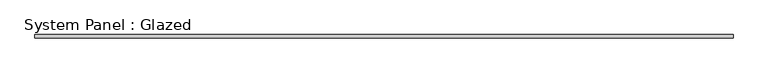
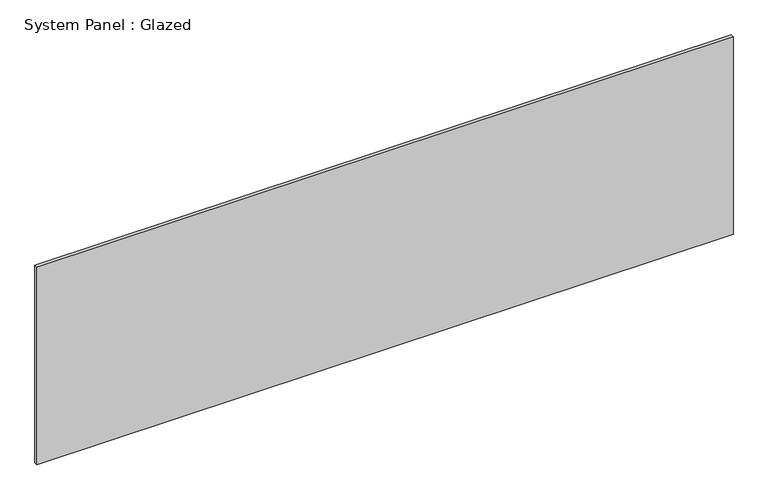
"""IFC4 building model written with IfcOpenShell, lengths in millimetres: plate geometry, System Panel : Glazed."""

from ifc_helpers import new_model, si_unit, origin, origin_with_axes, place, context, project, spatial, polyline, outline, extrude, source, transform, mapped, element, save


def system_panel_glazed_b7a52489(model_context):
    return source(origin(), model_context, "Body", "SweptSolid", [
        extrude(outline(polyline([(2540.0, 19.05), (-2540.0, 19.05), (-2540.0, 44.45), (2540.0, 44.45), (2540.0, 19.05)])), origin_with_axes(), (0.0, 0.0, 1.0), 1524.0),
    ])


if __name__ == "__main__":
    model = new_model("IFC4")
    model_context = context("Model", 3, world=origin())
    ifc_project = project(units=[si_unit("LENGTHUNIT", "METRE", prefix="MILLI")], contexts=[model_context])
    site = spatial("IfcSite", under=ifc_project)
    building = spatial("IfcBuilding", under=site)
    placement = place(None, origin())
    system_panel_glazed_shape = system_panel_glazed_b7a52489(model_context)
    element("IfcPlate", 1, ObjectType="System Panel : Glazed", at=placement, inside=building, context=model_context, shape_type="MappedRepresentation", body=[
        mapped(system_panel_glazed_shape, transform((0.0, 0.0, 0.0), x_axis=(1.0, 0.0, 0.0), y_axis=(0.0, 1.0, 0.0), z_axis=(0.0, 0.0, 1.0))),
    ])
    save(model, "model.ifc")

# Revit data of these elements
# Type "System Panel : Glazed"
#   Construction Type Id = "GSP4R"
#   Analytic Construction = "1/8 in Pilkington single glazing"
#   Visual Light Transmittance = 0.9
#   Solar Heat Gain Coefficient = 0.86
#   Heat Transfer Coefficient (U) = 1.18115 BTU/(h·ft²·°F)
# Element 1 (IfcPlate, "System Panel : Glazed")
#   Materials on its faces: "Glass"
# Materials
#   "Glass": class "Glass", colour RGB 0 128 192, transparency 0.75, Description = "Soda Lime Glass", Cost = 0
